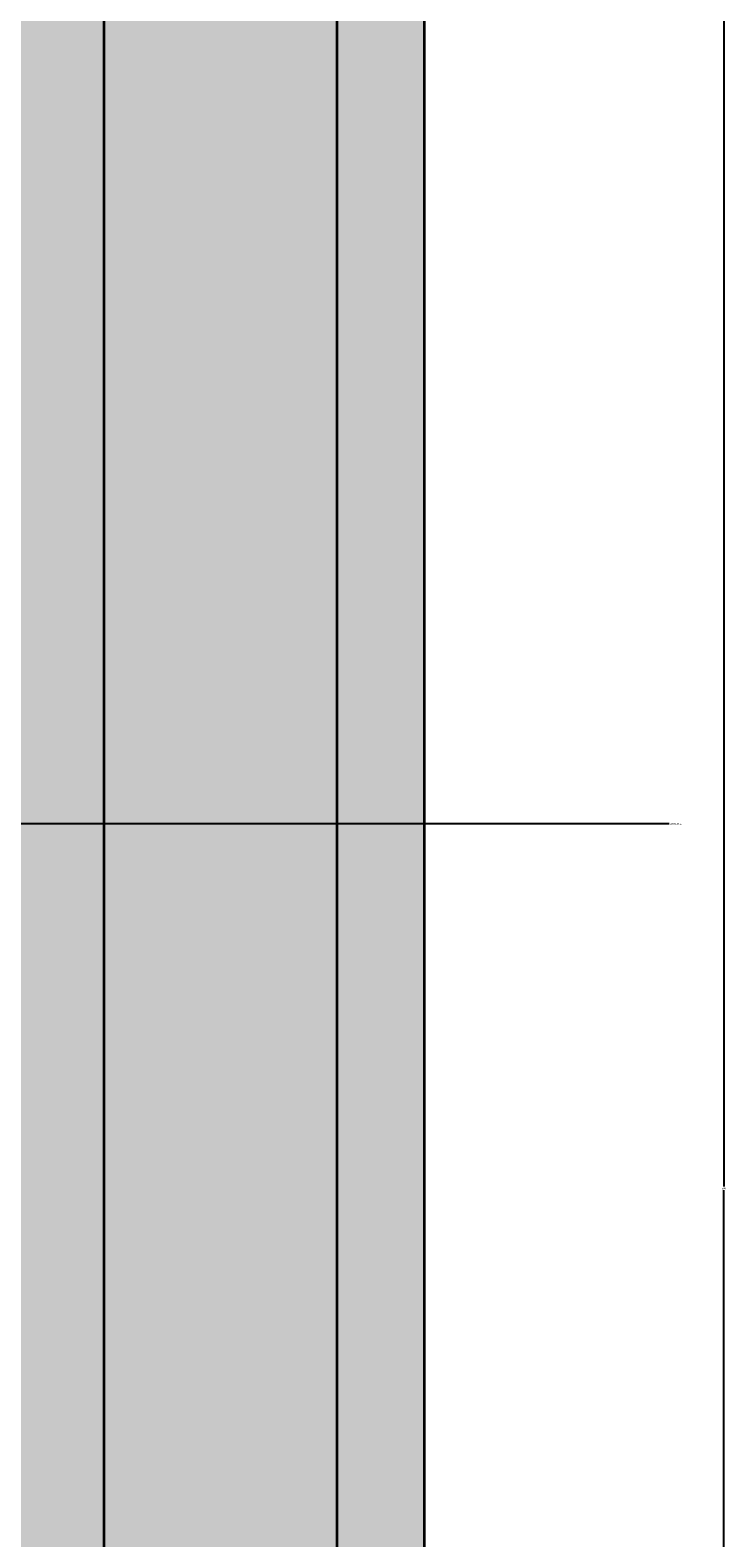
# Model space of a CAD drawing. Units: inches. Extents: x 2549 to 3108, y 1683 to 2362.
# Tile 29 of 30: x 3036 to 3108, y 1979 to 2134. Entities that reach past the tile are written whole.
import ezdxf

# ---------------------------------------------------------------- set-up
doc = ezdxf.new("R2010")
doc.units = ezdxf.units.IN
for name, color, linetype, lineweight in [('A-ANNO-DIMS', 2, 'Continuous', 18), ('A-WALL', 7, 'Continuous', 35), ('A-WALL-PATT', 89, 'Continuous', 13), ('C-PROP', 7, 'Continuous', 35)]:
    doc.layers.add(name, color=color, linetype=linetype, lineweight=lineweight)
doc.layers.add('C-PROP-PATT', color=252, linetype='Continuous', lineweight=13, true_color=0x939598)
doc.layers.add('C-PVMT-PATT', color=9, linetype='Continuous', lineweight=13, true_color=0xc7c8ca)
doc.styles.get("Standard").update_dxf_attribs({"font": 'arial.ttf'})
doc.dimstyles.get("Standard").update_dxf_attribs({"dimtxt": 0.18, "dimasz": 0.18, "dimexe": 0.18, "dimexo": 0.0625, "dimgap": 0.09, "dimtad": 0, "dimtih": 1, "dimtoh": 1, "dimdec": 4, "dimzin": 0, "dimdsep": 46, "dimtxsty": 'Standard', "dimcen": 0.09, "dimadec": 0, "dimazin": 0, "dimtfac": 1, "dimtdec": 4, "dimtofl": 0, "dimtmove": 0, "dimatfit": 3, "dimfxl": 1, "dimtolj": 1, "dimtzin": 0, "dimarcsym": 0})

# ---------------------------------------------------------------- blocks, each defined once
blk = doc.blocks.new('*D25')
at = {"layer": 'A-ANNO-DIMS', "color": 0, "lineweight": -2, "transparency": 16777216}
for p, q in [((3076.71, 2314.52), (3107.72, 2314.52)), ((3107.54, 2314.34), (3107.54, 2014.71)), ((3107.54, 1714.7), (3107.54, 2014.34)), ((3076.71, 1714.52), (3107.72, 1714.52))]:
    blk.add_line(p, q, dxfattribs=at)
at = {"layer": 'A-ANNO-DIMS', "color": 0, "transparency": 16777216}
for points in [[(3107.51, 2314.34), (3107.57, 2314.34), (3107.54, 2314.52)], [(3107.51, 1714.7), (3107.57, 1714.7), (3107.54, 1714.52)]]:
    blk.add_solid(points, dxfattribs=at)
at = {"layer": 'Defpoints', "color": 0, "transparency": 16777216}
for p in [(3076.64, 2314.52), (3107.54, 2314.52), (3076.64, 1714.52)]:
    blk.add_point(p, dxfattribs=at)
at = {"layer": 'A-ANNO-DIMS', "color": 0, "transparency": 16777216, "insert": (3107.54, 2014.52), "char_height": 0.18, "attachment_point": 5}
blk.add_mtext('\\A1;600', dxfattribs=at)
blk = doc.blocks.new('*D64')
at = {"layer": 'A-ANNO-DIMS', "color": 0, "lineweight": -2, "transparency": 16777216}
for p, q in [((2919.01, 2052.09), (2919.19, 2052.09)), ((2919.1, 2052), (2919.1, 2052.18)), ((3101.9, 2052.09), (3033.53, 2052.09))]:
    blk.add_line(p, q, dxfattribs=at)
at = {"layer": 'A-ANNO-DIMS', "color": 0, "transparency": 16777216}
blk.add_solid([(3033.53, 2052.12), (3033.53, 2052.06), (3033.35, 2052.09)], dxfattribs=at)
at = {"layer": 'Defpoints', "color": 0, "transparency": 16777216}
for p in [(2919.1, 2052.09), (3033.35, 2052.09)]:
    blk.add_point(p, dxfattribs=at)
at = {"layer": 'A-ANNO-DIMS', "color": 0, "transparency": 16777216, "insert": (3102.64, 2052.09), "char_height": 0.18, "attachment_point": 5}
blk.add_mtext('\\A1;2X R114.25', dxfattribs=at)

msp = doc.modelspace()

# ---------------------------------------------------------------- hatches: boundary and pattern name
at = {"layer": 'A-WALL-PATT'}
h = msp.add_hatch(color=256, dxfattribs=at)
h.dxf.hatch_style = 1
h.paths.add_polyline_path([(2638.6427, 2272.5237), (3034.6427, 2272.5237), (3034.6427, 1936.5237), (3043.6427, 1936.5237), (3043.6427, 2281.5237), (2629.6427, 2281.5237), (2629.6427, 2074.5237), (2812.6427, 2074.5237), (2812.6427, 2140.5237), (2785.7177, 2140.5237), (2785.7177, 2134.5237), (2806.6427, 2134.5237), (2806.6427, 2080.5237), (2638.6427, 2080.5237)])
h.paths.add_polyline_path([(2638.6427, 1972.5237), (2662.6427, 1972.5237), (2662.6427, 2041.0557), (2653.6427, 2041.0557), (2653.6427, 1978.5237), (2629.6427, 1978.5237), (2629.6427, 1795.5237), (2662.6427, 1795.5237), (2881.6427, 1795.5237), (2881.6427, 1936.5237), (2965.9351, 1936.5237), (2965.9351, 1974.5439), (2959.9351, 1974.5439), (2959.9351, 1945.5237), (2881.6427, 1945.5237), (2872.6427, 1945.5237), (2872.6427, 1804.5237), (2662.6427, 1804.5237), (2638.6427, 1804.5237)])
at = {"layer": 'C-PROP-PATT'}
h = msp.add_hatch(color=256, dxfattribs=at)
h.dxf.hatch_style = 1
h.paths.add_polyline_path([(3076.6427, 2314.5237), (2596.6427, 2314.5237), (2596.6427, 1714.5237), (2881.84, 1714.5237), (2881.84, 1723.5237), (2605.6427, 1723.5237), (2605.6427, 2305.5237), (3067.6427, 2305.5237), (3067.6427, 1723.5237), (3067.6427, 1714.5237), (3076.6427, 1714.5237)])
at = {"layer": 'C-PVMT-PATT'}
h = msp.add_hatch(color=256, dxfattribs=at)
h.dxf.hatch_style = 1
h.paths.add_polyline_path([(3067.6427, 2305.5237), (2605.6427, 2305.5237), (2605.6427, 2074.5237), (2629.6427, 2074.5237), (2629.6427, 2281.5237), (3043.6427, 2281.5237), (3043.6427, 1885.5237), (3043.6427, 1872.8745), (3031.1672, 1872.8745), (3031.1672, 1862.5731), (2995.8054, 1862.5731), (2995.8054, 1872.8745), (2983.1752, 1872.8745), (2983.1752, 1885.5237), (2881.6427, 1885.5237), (2881.6427, 1795.5237), (2751.0977, 1795.5237), (2751.0977, 1761.5237), (2786.1577, 1761.5237), (2786.1577, 1723.5237), (2881.84, 1723.5237), (2881.84, 1714.5237), (3067.6427, 1714.5237), (3067.6427, 1723.5237)])
edge = h.paths.add_edge_path(flags=16)
edge.add_ellipse((2949.4402, 1710.9683), major_axis=(-194.1014, 0), ratio=0.84230387, start_angle=-77.874034, end_angle=-76.219471, ccw=False)
edge.add_ellipse((2949.4402, 1715.2151), major_axis=(-189.1422, 0), ratio=0.84230387, start_angle=-79.790461, end_angle=-77.555373, ccw=False)
edge.add_ellipse((2899.9271, 2002.4692), major_axis=(155.4756, 0), ratio=0.84230387, start_angle=-80.743434, end_angle=-77.445067)
edge.add_line((2928.5915, 1873.7564), (2932.3882, 1875.8558))
edge.add_line((2932.3882, 1875.8558), (2936.1848, 1873.7564))
edge.add_ellipse((2964.8492, 2002.4692), major_axis=(-155.4756, 0), ratio=0.84230387, start_angle=77.445067, end_angle=80.743434)
edge.add_ellipse((2915.3361, 1715.2151), major_axis=(189.1422, 0), ratio=0.84230387, start_angle=77.555373, end_angle=79.790461, ccw=False)
edge.add_ellipse((2915.3361, 1710.9683), major_axis=(-194.1014, 0), ratio=0.84230387, start_angle=256.219471, end_angle=257.874034, ccw=False)
edge.add_ellipse((2628.2871, 1850.2612), major_axis=(-327.2532, 0), ratio=0.84230387, start_angle=182.17995, end_angle=183.650428, ccw=False)
edge.add_ellipse((2955.5637, 1861.9334), major_axis=(-0.9168, 0), ratio=0.84230387, start_angle=180, end_angle=270, ccw=False)
edge.add_line((2956.4805, 1862.3857), (2956.4805, 1846.4866))
edge.add_ellipse((2955.5637, 1846.939), major_axis=(-0.9168, 0), ratio=0.84230387, start_angle=90, end_angle=180, ccw=False)
edge.add_ellipse((-3607.0606, 1835.832), major_axis=(-6562.6242, 0), ratio=0.84230387, start_angle=179.61613322, end_angle=180.09022909, ccw=False)
edge.add_ellipse((2955.5637, 1791.0926), major_axis=(0.9168, 0), ratio=0.84230387, start_angle=0, end_angle=90, ccw=False)
edge.add_line((2956.4805, 1791.545), (2956.4805, 1775.6459))
edge.add_ellipse((2955.5637, 1776.0982), major_axis=(0.9168, 0), ratio=0.84230387, start_angle=270, end_angle=360, ccw=False)
edge.add_ellipse((-3607.0606, 1835.832), major_axis=(-6562.6242, 0), ratio=0.84230387, start_angle=179.3813568, end_angle=179.47172853, ccw=False)
edge.add_ellipse((2954.5907, 1763.8768), major_axis=(-1.3752, 0), ratio=0.84230387, start_angle=179.371763, end_angle=248.464757, ccw=False)
edge.add_ellipse((-3607.519, 1835.832), major_axis=(-6564.0409, 0), ratio=0.842303863, start_angle=179.35344594, end_angle=179.37176282, ccw=False)
edge.add_ellipse((2952.6829, 1761.8002), major_axis=(3.2503, 0), ratio=0.84230387, start_angle=-90, end_angle=-0.646554, ccw=False)
edge.add_line((2952.6829, 1759.0625), (2912.0934, 1759.0625))
edge.add_ellipse((2912.0934, 1761.8002), major_axis=(3.2503, 0), ratio=0.84230387, start_angle=180.646554, end_angle=270, ccw=False)
edge.add_ellipse((9472.2953, 1835.832), major_axis=(-6564.0409, 0), ratio=0.842303871, start_angle=0.62823722, end_angle=0.6465541, ccw=False)
edge.add_ellipse((2910.1856, 1763.8768), major_axis=(1.3752, 0), ratio=0.84230387, start_angle=111.535244, end_angle=180.628237, ccw=False)
edge.add_ellipse((9471.8369, 1835.832), major_axis=(-6562.6242, 0), ratio=0.84230387, start_angle=0.52827147, end_angle=0.6465541, ccw=False)
edge.add_ellipse((2909.2126, 1776.0982), major_axis=(-0.9168, 0), ratio=0.84230387, start_angle=0, end_angle=90, ccw=False)
edge.add_line((2908.2958, 1775.6459), (2908.2958, 1791.545))
edge.add_ellipse((2909.2126, 1791.0926), major_axis=(-0.9168, 0), ratio=0.84230387, start_angle=-90, end_angle=0, ccw=False)
edge.add_ellipse((9471.8369, 1835.832), major_axis=(-6562.6242, 0), ratio=0.84230387, start_angle=-0.09022909, end_angle=0.38386678, ccw=False)
edge.add_ellipse((2909.2126, 1846.939), major_axis=(-0.9168, 0), ratio=0.84230387, start_angle=0, end_angle=90, ccw=False)
edge.add_line((2908.2958, 1846.4866), (2908.2958, 1862.3857))
edge.add_ellipse((2909.2126, 1861.9334), major_axis=(0.9168, 0), ratio=0.84230387, start_angle=90, end_angle=180, ccw=False)
edge.add_ellipse((3236.4892, 1850.2612), major_axis=(327.2532, 0), ratio=0.84230387, start_angle=176.349572, end_angle=177.82005, ccw=False)
edge = h.paths.add_edge_path(flags=0)
edge.add_ellipse((2903.4793, 1857.3351), major_axis=(-34.7979, 0), ratio=0.84230387, start_angle=180, end_angle=209.43857, ccw=False)
edge.add_line((2938.2772, 1857.3351), (2938.2772, 1855.8792))
edge.add_line((2938.2772, 1855.8792), (2939.4631, 1855.8792))
edge.add_line((2939.4631, 1855.8792), (2943.0251, 1853.3975))
edge.add_line((2943.0251, 1853.3975), (2943.0251, 1844.2222))
edge.add_ellipse((2940.6512, 1844.3143), major_axis=(0.2209, 3.9278), ratio=0.60383358, start_angle=106.342592, end_angle=270.997986, ccw=False)
edge.add_line((2938.2772, 1843.7609), (2938.2772, 1857.3351))
edge.add_ellipse((2903.4793, 1857.3351), major_axis=(-34.7979, 0), ratio=0.84230387, start_angle=180, end_angle=209.43857)
edge.add_ellipse((2961.297, 1857.3351), major_axis=(34.7979, 0), ratio=0.84230387, start_angle=150.56143, end_angle=180)
edge.add_line((2926.4991, 1857.3351), (2926.4991, 1843.7609))
edge.add_ellipse((2924.1251, 1844.3143), major_axis=(-0.2209, 3.9278), ratio=0.60383358, start_angle=89.002014, end_angle=253.657408, ccw=False)
edge.add_line((2921.7512, 1844.2222), (2921.7512, 1853.3975))
edge.add_line((2921.7512, 1853.3975), (2925.3132, 1855.8792))
edge.add_line((2925.3132, 1855.8792), (2926.4991, 1855.8792))
edge.add_line((2926.4991, 1855.8792), (2926.4991, 1857.3351))
edge.add_ellipse((2961.297, 1857.3351), major_axis=(34.7979, 0), ratio=0.84230387, start_angle=150.56143, end_angle=180, ccw=False)
edge = h.paths.add_edge_path(flags=0)
edge.add_ellipse((2929.0505, 1791.964), major_axis=(50.66, 0), ratio=0.84230387, start_angle=94.277421, end_angle=111.834954, ccw=False)
edge.add_line((2925.8653, 1834.5507), (2938.911, 1834.5507))
edge.add_ellipse((2935.7258, 1791.964), major_axis=(-50.66, 0), ratio=0.84230387, start_angle=248.165046, end_angle=265.722579, ccw=False)
edge.add_line((2951.9255, 1832.3947), (2950.5719, 1822.2495))
edge.add_ellipse((2934.1225, 1783.1023), major_axis=(49.3014, 0), ratio=0.84230387, start_angle=67.208085, end_angle=85.12993)
edge.add_line((2937.6516, 1824.5225), (2927.1247, 1824.5225))
edge.add_ellipse((2930.6538, 1783.1023), major_axis=(-49.3014, 0), ratio=0.84230387, start_angle=-85.12993, end_angle=-67.208085)
edge.add_line((2914.2044, 1822.2495), (2912.8508, 1832.3947))
edge = h.paths.add_edge_path(flags=0)
edge.add_line((2910.1338, 1829.4651), (2912.6432, 1821.2711))
edge.add_ellipse((5203.7787, 1816.4367), major_axis=(-2291.1426, 0), ratio=0.84230387, start_angle=-0.1208974, end_angle=0.3640763)
edge.add_line((2912.7012, 1801.8782), (2910.3305, 1792.5698))
edge.add_ellipse((9471.8369, 1835.832), major_axis=(-6561.7074, 0), ratio=0.84230387, start_angle=0.05559431, end_angle=0.37776419, ccw=False)
edge = h.paths.add_edge_path(flags=0)
edge.add_ellipse((-3607.0606, 1835.832), major_axis=(6561.7074, 0), ratio=0.84230387, start_angle=-0.37776419, end_angle=-0.05559431, ccw=False)
edge.add_line((2954.4458, 1792.5698), (2952.0751, 1801.8782))
edge.add_ellipse((660.9976, 1816.4367), major_axis=(2291.1426, 0), ratio=0.84230387, start_angle=-0.3640763, end_angle=0.1208974)
edge.add_line((2952.1331, 1821.2711), (2954.6425, 1829.4651))
edge = h.paths.add_edge_path(flags=0)
edge.add_ellipse((2932.3882, 1865.1973), major_axis=(91.081, 0), ratio=0.84230387, start_angle=256.401865, end_angle=283.598135)
edge.add_line((2950.5719, 1790.0239), (2950.5719, 1778.3622))
edge.add_ellipse((2932.3882, 1853.5356), major_axis=(91.081, 0), ratio=0.84230387, start_angle=256.401865, end_angle=283.598135, ccw=False)
edge.add_line((2914.2044, 1778.3622), (2914.2044, 1790.0239))
edge = h.paths.add_edge_path(flags=0)
edge.add_line((2916.038, 1773.859), (2948.7383, 1773.859))
edge.add_ellipse((2948.7383, 1772.3145), major_axis=(1.8336, 0), ratio=0.84230387, start_angle=0, end_angle=90, ccw=False)
edge.add_line((2950.5719, 1772.3145), (2950.5719, 1760.2558))
edge.add_line((2950.5719, 1760.2558), (2914.2044, 1760.2558))
edge.add_line((2914.2044, 1760.2558), (2914.2044, 1772.3145))
edge.add_ellipse((2916.038, 1772.3145), major_axis=(1.8336, 0), ratio=0.84230387, start_angle=90, end_angle=180, ccw=False)
h.paths.add_polyline_path([(2629.6427, 1978.5237), (2605.6427, 1978.5237), (2605.6427, 1723.5237), (2629.6427, 1723.5237), (2629.6427, 1795.5237)], flags=17)
h.paths.add_polyline_path([(2800.5245, 1759.1674), (2853.7435, 1759.1674), (2853.7435, 1768.954), (2800.5245, 1768.954)], flags=24)
h.paths.add_polyline_path([(2972.4611, 1807.3305), (3015.3943, 1807.3305), (3015.3943, 1817.117), (2972.4611, 1817.117)], flags=24)

# ---------------------------------------------------------------- linework, layer by layer
at = {"layer": 'A-WALL'}
msp.add_line((3043.6427, 2281.5237), (3043.6427, 1885.5237), dxfattribs=at)
at = {"layer": 'C-PROP'}
msp.add_lwpolyline([(2596.6427, 2314.5237), (3076.6427, 2314.5237), (3076.6427, 1714.5237), (2596.6427, 1714.5237)], close=True, dxfattribs=at)
msp.add_lwpolyline([(2881.84, 1723.5237), (2605.6427, 1723.5237), (2605.6427, 2305.5237), (3067.6427, 2305.5237), (3067.6427, 1723.5237)], dxfattribs=at)

# ---------------------------------------------------------------- dimensions: what is measured, and where the dimension line sits
at = {"layer": 'A-ANNO-DIMS'}
dim = msp.add_linear_dim(base=(3107.5427, 2314.5237), p1=(3076.6427, 1714.5237), p2=(3076.6427, 2314.5237), angle=90, dimstyle='Standard', override={"dimdec": 0, "dimlfac": 1, "dimrnd": 0, "dimzin": 0, "dimdsep": 46, "dimlunit": 2}, dxfattribs=at)
dim.commit()
dim.dimension.update_dxf_attribs({"geometry": '*D25', "text_midpoint": (3107.5427, 2014.5237)})
dim = msp.add_radius_dim(center=(2919.097, 2052.0905), mpoint=(3033.347, 2052.091), text='2X <>', dimstyle='Standard', override={"dimdec": 2, "dimlfac": 1, "dimrnd": 0, "dimzin": 0, "dimdsep": 46, "dimlunit": 2}, dxfattribs=at)
dim.commit()
dim.dimension.update_dxf_attribs({"geometry": '*D64', "text_midpoint": (3101.897, 2052.0913), "dimtype": 164})

doc.saveas('drawing.dxf')
